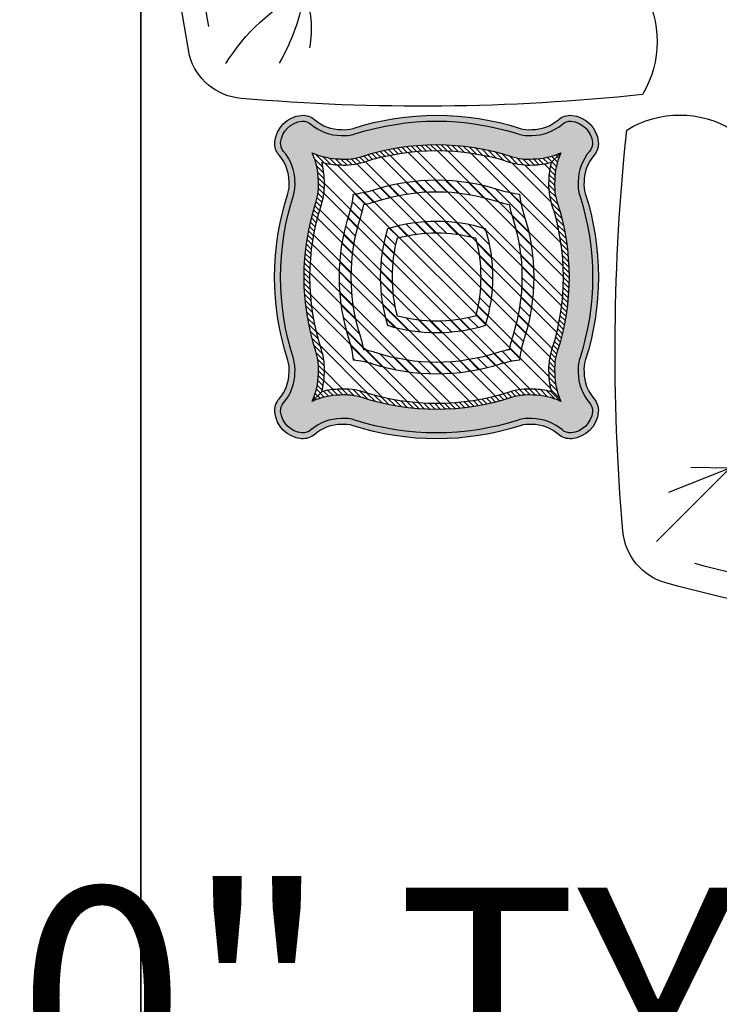
# Model space of a CAD drawing. Units: inches. Extents: x 844 to 2234, y 346 to 1084.
# Tile 5 of 93: x 1093 to 1112, y 653 to 680. Entities that reach past the tile are written whole.
import ezdxf

# ---------------------------------------------------------------- set-up
doc = ezdxf.new("R2010")
doc.units = ezdxf.units.IN
doc.header["$MEASUREMENT"] = 0
for name, color, linetype, lineweight in [('A-ANNO-DIMS', 2, 'Continuous', 18), ('A-WALL', 7, 'Continuous', 35), ('furniture', 8, 'Continuous', 18)]:
    doc.layers.add(name, color=color, linetype=linetype, lineweight=lineweight)
for name, color, linetype in [('RA-AP-01$0$FURN', 3, 'Continuous'), ('RA-AP-01$0$steel', 193, 'Continuous'), ('RA-AP-01$0$WOOD', 64, 'Continuous')]:
    doc.layers.add(name, color=color, linetype=linetype)
doc.styles.get("Standard").update_dxf_attribs({"font": 'arial.ttf'})
doc.dimstyles.get("Standard").update_dxf_attribs({"dimtxt": 6, "dimasz": 3, "dimexe": 0.18, "dimexo": 0.0625, "dimgap": 0.09, "dimtad": 0, "dimtih": 1, "dimtoh": 1, "dimdec": 1, "dimzin": 0, "dimdsep": 46, "dimlunit": 3, "dimtxsty": 'Standard', "dimblk": 'ARCHTICK', "dimcen": 0.09, "dimadec": 0, "dimazin": 0, "dimtfac": 1, "dimtdec": 1, "dimtofl": 0, "dimtmove": 0, "dimatfit": 3, "dimfxl": 1, "dimtolj": 1, "dimtzin": 0, "dimarcsym": 0})
pattern_1 = [(45, (0, 1.362436106329781), (-0.0088388347648318, 0.0088388347648318), [])]
pattern_2 = [(45, (0, 1.362436106329781), (-0.0044194173824159, 0.0044194173824159), [])]

# ---------------------------------------------------------------- blocks, each defined once
blk = doc.blocks.new('A$C2FCF5309')
at = {"layer": 'RA-AP-01$0$FURN'}
h = blk.add_hatch(dxfattribs=at)
h.set_pattern_fill('ANSI31', color=256, scale=0.1, style=0)
h.set_pattern_definition(pattern_1)
h.paths.add_polyline_path([(5.038683893313746, -5.169250834004607, -0.1583983521602212), (5.038683893312098, -5.373464580902012, 0.0306258898943267), (5.033304057242972, -5.394827569605182, 0.0306258898948892), (5.01194106853941, -5.40020740567441, -0.1028142994996694), (4.878286182323899, -5.414871334512708), (4.863600873530158, -5.43331743520547, 0.1120482678681049), (5.018059823131753, -5.419248541734471, -0.052642197802937), (5.050972078299936, -5.412495590662115, -0.0526421977994963), (5.057725029371615, -5.379583335496025, 0.1583028414702701), (5.057725029372958, -5.163132079409654, -0.052642197806903), (5.050972078299777, -5.130219824239078, -0.0526421977995126), (5.018059823133679, -5.123466873167369, 0.0215995840215353), (4.988903013548211, -5.115372132362452), (4.975007495303644, -5.132826183367946, -0.0289147572844802), (5.011941068537408, -5.142508009226167, 0.0306258898976746), (5.033304057242868, -5.147887845296027, 0.0306258899022411)])
h.paths.add_polyline_path([(4.975007495303645, -5.132826183367946), (4.988903013548211, -5.115372132362452, 0.1362374241599938), (4.801608567045604, -5.12346687316654, -0.0526421978036853), (4.768696311876971, -5.130219824239102, -0.05264219780204), (4.761943360804856, -5.163132079406747, 0.1583028414743723), (4.761943360806116, -5.379583335498449, -0.0526421977955461), (4.768696311877141, -5.412495590662114, -0.0526421978073986), (4.801608567048022, -5.419248541735437, 0.0454484293938888), (4.863600873530158, -5.43331743520547), (4.878286182323899, -5.414871334512708, -0.0546933379798044), (4.80772732164382, -5.40020740567649, 0.030625889903973), (4.786364332934043, -5.394827569605216, 0.0306258898932853), (4.780984496865101, -5.373464580902791, -0.1583983521638281), (4.780984496864308, -5.169250834000963, 0.03062588989692), (4.786364332933943, -5.147887845296004, 0.0306258898946324), (4.807727321637318, -5.142508009226805, -0.1288932573266927)])
h.paths.add_polyline_path([(4.843422214712861, -5.204945727074827, -0.0783685831716868), (4.924134454130224, -5.196727409635105), (4.939146578618322, -5.177870798323143, 0.1012675676854134), (4.827248748758957, -5.188772261120899, 0.1253648873081696), (4.820394258584192, -5.327034652050361), (4.837127701354095, -5.306015906404253, -0.0981593964869636)], flags=17)
h.paths.add_polyline_path([(4.843422214712824, -5.337769687826355, -0.0311091841722656), (4.837127701354095, -5.306015906404253), (4.820394258584193, -5.32703465205036, 0.0247727657431944), (4.827248748758908, -5.353943153780261, 0.0812754385032542), (4.916962478476905, -5.36629034358622), (4.933684093813825, -5.345286454285511, -0.0876255421014372)], flags=17)
h.paths.add_polyline_path([(4.992419641418037, -5.353943153780226, 0.1506053783834298), (4.992419641417933, -5.188772261120954, 0.0485966419124224), (4.939146578618321, -5.177870798323143), (4.924134454130224, -5.196727409635105, -0.0507799419579301), (4.976246175464031, -5.204945727074882, -0.1296645318906876), (4.97624617546411, -5.337769687826316, -0.0415667119298777), (4.933684093813825, -5.345286454285511), (4.916962478476905, -5.36629034358622, 0.0684915676023693)], flags=17)
h = blk.add_hatch(dxfattribs=at)
h.set_pattern_fill('ANSI31', color=256, scale=0.1, style=0)
h.set_pattern_definition(pattern_1)
h.paths.add_polyline_path([(5.038683893313746, -5.169250834004607, -0.1583983521602212), (5.038683893312098, -5.373464580902012, 0.0306258898943267), (5.033304057242972, -5.394827569605182, 0.0306258898948892), (5.01194106853941, -5.40020740567441, -0.1028142994996694), (4.878286182323899, -5.414871334512708), (4.863600873530158, -5.43331743520547, 0.1120482678681049), (5.018059823131753, -5.419248541734471, -0.052642197802937), (5.050972078299936, -5.412495590662115, -0.0526421977994963), (5.057725029371615, -5.379583335496025, 0.1583028414702701), (5.057725029372958, -5.163132079409654, -0.052642197806903), (5.050972078299777, -5.130219824239078, -0.0526421977995126), (5.018059823133679, -5.123466873167369, 0.0215995840215353), (4.988903013548211, -5.115372132362452), (4.975007495303644, -5.132826183367946, -0.0289147572844802), (5.011941068537408, -5.142508009226167, 0.0306258898976746), (5.033304057242868, -5.147887845296027, 0.0306258899022411)])
h.paths.add_polyline_path([(4.975007495303645, -5.132826183367946), (4.988903013548211, -5.115372132362452, 0.1362374241599938), (4.801608567045604, -5.12346687316654, -0.0526421978036853), (4.768696311876971, -5.130219824239102, -0.05264219780204), (4.761943360804856, -5.163132079406747, 0.1583028414743723), (4.761943360806116, -5.379583335498449, -0.0526421977955461), (4.768696311877141, -5.412495590662114, -0.0526421978073986), (4.801608567048022, -5.419248541735437, 0.0454484293938888), (4.863600873530158, -5.43331743520547), (4.878286182323899, -5.414871334512708, -0.0546933379798044), (4.80772732164382, -5.40020740567649, 0.030625889903973), (4.786364332934043, -5.394827569605216, 0.0306258898932853), (4.780984496865101, -5.373464580902791, -0.1583983521638281), (4.780984496864308, -5.169250834000963, 0.03062588989692), (4.786364332933943, -5.147887845296004, 0.0306258898946324), (4.807727321637318, -5.142508009226805, -0.1288932573266927)])
h.paths.add_polyline_path([(4.843422214712861, -5.204945727074827, -0.0783685831716868), (4.924134454130224, -5.196727409635105), (4.939146578618322, -5.177870798323143, 0.1012675676854134), (4.827248748758957, -5.188772261120899, 0.1253648873081696), (4.820394258584192, -5.327034652050361), (4.837127701354095, -5.306015906404253, -0.0981593964869636)], flags=17)
h.paths.add_polyline_path([(4.843422214712824, -5.337769687826355, -0.0311091841722656), (4.837127701354095, -5.306015906404253), (4.820394258584193, -5.32703465205036, 0.0247727657431944), (4.827248748758908, -5.353943153780261, 0.0812754385032542), (4.916962478476905, -5.36629034358622), (4.933684093813825, -5.345286454285511, -0.0876255421014372)], flags=17)
h.paths.add_polyline_path([(4.992419641418037, -5.353943153780226, 0.1506053783834298), (4.992419641417933, -5.188772261120954, 0.0485966419124224), (4.939146578618321, -5.177870798323143), (4.924134454130224, -5.196727409635105, -0.0507799419579301), (4.976246175464031, -5.204945727074882, -0.1296645318906876), (4.97624617546411, -5.337769687826316, -0.0415667119298777), (4.933684093813825, -5.345286454285511), (4.916962478476905, -5.36629034358622, 0.0684915676023693)], flags=17)
at = {"layer": 'RA-AP-01$0$WOOD'}
h = blk.add_hatch(color=256, dxfattribs=at)
edge = h.paths.add_edge_path()
edge.add_arc((4.683001772622394, -5.026441828662609), 0.0299999999999998, 48.77105092035535, 95.25687599427813)
edge.add_arc((4.684834195088484, -5.046357707450686), 0.0499999999998897, 95.25687599443106, 174.7431240064049)
edge.add_arc((4.664918316300367, -5.044525284985046), 0.0300000000000005, 174.7431240062535, 221.2289490796905)
edge.add_arc((4.591236830209155, -5.109094338216345), 0.0679700159630267, -0.5333070513215148, 41.228949079691915, ccw=False)
edge.add_arc((4.609451302807284, -5.114694777173187), 0.0500000000000008, -17.3556839752095, 5.7020707654044145, ccw=False)
edge.add_arc((5.095208119646659, -5.271357707450659), 0.4603971832811796, 162.0683908477609, 197.9316091523306)
edge.add_arc((4.609451302807533, -5.428020637728902), 0.0500000000000006, -5.702070765320514, 17.355683975293914, ccw=False)
edge.add_arc((4.591236830209412, -5.433621076685779), 0.0679700159630261, -41.228949079600625, 0.5333070514128053, ccw=False)
edge.add_arc((4.664918316300727, -5.498190129916959), 0.0299999999999995, 138.7710509204022, 185.256875994324)
edge.add_arc((4.684834195088642, -5.496357707450695), 0.0499999999997451, 185.2568759946742, 264.74312400432)
edge.add_arc((4.683001772622394, -5.516273586238612), 0.03, 264.743124003969, 311.2289490796446)
edge.add_arc((4.747570825853633, -5.589955072329876), 0.0679700159630271, 89.4666929486321, 131.2289490796457, ccw=False)
edge.add_arc((4.753171264810493, -5.57174059973175), 0.0500000000000015, 72.64431602474701, 95.70207076536133, ccw=False)
edge.add_arc((4.909834195088355, -5.085983782892503), 0.4603971832811774, 252.0683908477147, 287.9316091522845)
edge.add_arc((5.06649712536621, -5.57174059973175), 0.0499999999999999, 84.29792923463953, 107.35568397525361, ccw=False)
edge.add_arc((5.072097564323069, -5.589955072329877), 0.0679700159630274, 48.771050920354185, 90.5333070513679, ccw=False)
edge.add_arc((5.136666617554309, -5.516273586238614), 0.0299999999999997, 228.771050920353, 275.2568759942969)
edge.add_arc((5.134834195088338, -5.496357707450417), 0.0499999999999982, 275.2568759942949, 354.7431240057633)
edge.add_arc((5.154750073876535, -5.498190129916372), 0.0299999999999999, 354.7431240057662, 401.2289490796891)
edge.add_arc((5.228431559967749, -5.433621076685074), 0.0679700159630274, 179.4666929486771, 221.2289490796903, ccw=False)
edge.add_arc((5.210217087369615, -5.428020637728227), 0.0499999999999976, 162.6443160247947, 185.7020707654089, ccw=False)
edge.add_arc((4.724460270530244, -5.271357707450757), 0.4603971832811793, 342.0683908477607, 377.9316091523305)
edge.add_arc((5.210217087369368, -5.114694777172509), 0.0500000000000019, 174.2979292346878, 197.355683975302, ccw=False)
edge.add_arc((5.228431559967489, -5.109094338215639), 0.0679700159630279, 138.7710509203993, 180.5333070514128, ccw=False)
edge.add_arc((5.154750073876174, -5.044525284984457), 0.0300000000000001, 318.771050920401, 365.2568759954636)
edge.add_arc((5.13483419508816, -5.046357707450624), 0.0499999999998349, 5.256875995237118, 84.74312400549572)
edge.add_arc((5.136666617554308, -5.026441828662608), 0.0299999999999994, 84.74312400572185, 131.2289490796446)
edge.add_arc((5.072097564323072, -4.952760342571343), 0.0679700159630261, 269.4666929486298, 311.22894907964354, ccw=False)
edge.add_arc((5.066497125366206, -4.97097481516947), 0.0499999999999992, 252.64431602475162, 275.70207076536565, ccw=False)
edge.add_arc((4.909834195088355, -5.456731632008717), 0.4603971832811764, 72.06839084771546, 107.9316091522853)
edge.add_arc((4.753171264810493, -4.970974815169471), 0.0500000000000016, 264.2979292346387, 287.355683975253, ccw=False)
edge.add_arc((4.747570825853633, -4.952760342571346), 0.0679700159630274, 228.7710509203543, 270.5333070513679, ccw=False)
edge = h.paths.add_edge_path(flags=16)
edge.add_arc((4.683001772622395, -5.026441828662608), 0.019999999999999, 48.7710509203555, 95.2568759942793)
edge.add_arc((4.684834195088469, -5.046357707450671), 0.0399999999998731, 95.2568759944489, 174.7431240064248)
edge.add_arc((4.664918316300404, -5.044525284985035), 0.020000000000036, 174.7431240062186, 221.2289490796461)
edge.add_arc((4.591236830209151, -5.109094338216346), 0.0779700159630296, -0.13764630038667747, 41.228949079689585, ccw=False)
edge.add_arc((4.609451302807307, -5.11469477717304), 0.060000000000024, -17.406127045137907, 5.176192161068002, ccw=False)
edge.add_arc((5.09520811964665, -5.271357707450659), 0.4503971832811708, 162.0623235129628, 197.9376764869162)
edge.add_arc((4.609451302807532, -5.428020637728943), 0.0599999999999982, -5.176192160466428, 17.406127046715312, ccw=False)
edge.add_arc((4.591236830209414, -5.433621076685778), 0.0779700159630257, -41.2289490796029, 0.13764630095249686, ccw=False)
edge.add_arc((4.664918316300731, -5.498190129916961), 0.0200000000000047, 138.7710509204103, 185.2568759943212)
edge.add_arc((4.684834195088606, -5.496357707450731), 0.0399999999997066, 185.2568759947174, 264.7431240043665)
edge.add_arc((4.683001772622369, -5.516273586238541), 0.020000000000069, 264.7431240038842, 311.2289490795622)
edge.add_arc((4.747570825853635, -5.589955072329884), 0.0779700159630344, 89.8623536987642, 131.2289490796432, ccw=False)
edge.add_arc((4.753171264810603, -5.571740599731771), 0.0599999999999895, 72.5938729544394, 95.1761921602253, ccw=False)
edge.add_arc((4.909834195088365, -5.085983782892505), 0.4503971832811724, 252.0623235129989, 287.9376764870498)
edge.add_arc((5.066497125366216, -5.571740599731755), 0.0600000000000047, 84.8238078399923, 107.40612704528041, ccw=False)
edge.add_arc((5.072097564322998, -5.589955072329853), 0.077970015963056, 48.771050920303594, 90.13764630126451, ccw=False)
edge.add_arc((5.136666617554307, -5.516273586238622), 0.0199999999999931, 228.771050920344, 275.2568759943037)
edge.add_arc((5.134834195088338, -5.496357707450416), 0.0400000000000004, 275.2568759942928, 354.7431240057607)
edge.add_arc((5.154750073876533, -5.498190129916375), 0.0200000000000037, 354.7431240057783, 401.2289490796939)
edge.add_arc((5.228431559967745, -5.433621076685076), 0.0779700159630239, 179.8623536995147, 221.2289490796908, ccw=False)
edge.add_arc((5.210217087369586, -5.428020637728345), 0.0600000000000054, 162.5938729554486, 185.1761921609759, ccw=False)
edge.add_arc((4.724460270530243, -5.271357707450766), 0.4503971832811826, 342.0623235128896, 377.937676486982)
edge.add_arc((5.210217087369347, -5.114694777172486), 0.0599999999999777, 174.8238078387611, 197.4061270462219, ccw=False)
edge.add_arc((5.228431559967523, -5.109094338215542), 0.0779700159629885, 138.7710509204687, 180.1376463004423, ccw=False)
edge.add_arc((5.154750073876175, -5.044525284984459), 0.0199999999999989, 318.771050920406, 365.2568759954698)
edge.add_arc((5.134834195088138, -5.046357707450646), 0.0399999999998586, 5.256875995208452, 84.74312400546732)
edge.add_arc((5.136666617554292, -5.02644182866256), 0.0199999999999529, 84.74312400577769, 131.2289490797025)
edge.add_arc((5.072097564323069, -4.952760342571338), 0.077970015963032, 269.86235369901414, 311.2289490796421, ccw=False)
edge.add_arc((5.06649712536618, -4.97097481516946), 0.0600000000000007, 252.5938729548277, 275.17619216047467, ccw=False)
edge.add_arc((4.909834195088353, -5.456731632008716), 0.4503971832811739, 72.06232351293887, 107.9376764867365)
edge.add_arc((4.753171264810429, -4.970974815169467), 0.0599999999999991, 264.82380783985815, 287.40612704769893, ccw=False)
edge.add_arc((4.747570825853681, -4.952760342571361), 0.0779700159630467, 228.7710509203206, 270.13764630113724, ccw=False)
h = blk.add_hatch(color=256, dxfattribs=at)
edge = h.paths.add_edge_path()
edge.add_arc((4.683001772622395, -5.026441828662608), 0.019999999999999, 48.7710509203555, 95.2568759942793)
edge.add_arc((4.684834195088469, -5.046357707450671), 0.0399999999998731, 95.2568759944489, 174.7431240064248)
edge.add_arc((4.664918316300404, -5.044525284985035), 0.020000000000036, 174.7431240062186, 221.2289490796461)
edge.add_arc((4.591236830209151, -5.109094338216346), 0.0779700159630296, -0.13764630038667747, 41.228949079689585, ccw=False)
edge.add_arc((4.609451302807307, -5.11469477717304), 0.060000000000024, -17.406127045137907, 5.176192161068002, ccw=False)
edge.add_arc((5.09520811964665, -5.271357707450659), 0.4503971832811708, 162.0623235129628, 197.9376764869162)
edge.add_arc((4.609451302807532, -5.428020637728943), 0.0599999999999982, -5.176192160466428, 17.406127046715312, ccw=False)
edge.add_arc((4.591236830209414, -5.433621076685778), 0.0779700159630257, -41.2289490796029, 0.13764630095249686, ccw=False)
edge.add_arc((4.664918316300731, -5.498190129916961), 0.0200000000000047, 138.7710509204103, 185.2568759943212)
edge.add_arc((4.684834195088606, -5.496357707450731), 0.0399999999997066, 185.2568759947174, 264.7431240043665)
edge.add_arc((4.683001772622369, -5.516273586238541), 0.020000000000069, 264.7431240038842, 311.2289490795622)
edge.add_arc((4.747570825853635, -5.589955072329884), 0.0779700159630344, 89.8623536987642, 131.2289490796432, ccw=False)
edge.add_arc((4.753171264810603, -5.571740599731771), 0.0599999999999895, 72.5938729544394, 95.1761921602253, ccw=False)
edge.add_arc((4.909834195088365, -5.085983782892505), 0.4503971832811724, 252.0623235129989, 287.9376764870498)
edge.add_arc((5.066497125366216, -5.571740599731755), 0.0600000000000047, 84.8238078399923, 107.40612704528041, ccw=False)
edge.add_arc((5.072097564322998, -5.589955072329853), 0.077970015963056, 48.771050920303594, 90.13764630126451, ccw=False)
edge.add_arc((5.136666617554307, -5.516273586238622), 0.0199999999999931, 228.771050920344, 275.2568759943037)
edge.add_arc((5.134834195088338, -5.496357707450416), 0.0400000000000004, 275.2568759942928, 354.7431240057607)
edge.add_arc((5.154750073876533, -5.498190129916375), 0.0200000000000037, 354.7431240057783, 401.2289490796939)
edge.add_arc((5.228431559967745, -5.433621076685076), 0.0779700159630239, 179.8623536995147, 221.2289490796908, ccw=False)
edge.add_arc((5.210217087369586, -5.428020637728345), 0.0600000000000054, 162.5938729554486, 185.1761921609759, ccw=False)
edge.add_arc((4.724460270530243, -5.271357707450766), 0.4503971832811826, 342.0623235128896, 377.937676486982)
edge.add_arc((5.210217087369347, -5.114694777172486), 0.0599999999999777, 174.8238078387611, 197.4061270462219, ccw=False)
edge.add_arc((5.228431559967523, -5.109094338215542), 0.0779700159629885, 138.7710509204687, 180.1376463004423, ccw=False)
edge.add_arc((5.154750073876175, -5.044525284984459), 0.0199999999999989, 318.771050920406, 365.2568759954698)
edge.add_arc((5.134834195088138, -5.046357707450646), 0.0399999999998586, 5.256875995208452, 84.74312400546732)
edge.add_arc((5.136666617554292, -5.02644182866256), 0.0199999999999529, 84.74312400577769, 131.2289490797025)
edge.add_arc((5.072097564323069, -4.952760342571338), 0.077970015963032, 269.86235369901414, 311.2289490796421, ccw=False)
edge.add_arc((5.06649712536618, -4.97097481516946), 0.0600000000000007, 252.5938729548277, 275.17619216047467, ccw=False)
edge.add_arc((4.909834195088353, -5.456731632008716), 0.4503971832811739, 72.06232351293887, 107.9376764867365)
edge.add_arc((4.753171264810429, -4.970974815169467), 0.0599999999999991, 264.82380783985815, 287.40612704769893, ccw=False)
edge.add_arc((4.747570825853681, -4.952760342571361), 0.0779700159630467, 228.7710509203206, 270.13764630113724, ccw=False)
edge = h.paths.add_edge_path(flags=16)
edge.add_arc((4.591236830209151, -5.109094338216348), 0.1179700159630308, 0.7417751874182841, 24.563326950263672, ccw=False)
edge.add_arc((4.609451302807302, -5.114694777173093), 0.100000000000012, -17.52836504564658, 4.087328884225087, ccw=False)
edge.add_arc((5.095208119646651, -5.271357707450657), 0.4103971832811724, 162.0403002448777, 197.9596997550675)
edge.add_arc((4.60945130280753, -5.428020637728918), 0.1000000000000027, -4.087328883827581, 17.528365046291924, ccw=False)
edge.add_arc((4.591236830209414, -5.433621076685779), 0.1179700159630246, 335.43667305041845, 359.2582248129738, ccw=False)
edge.add_arc((4.747570825853596, -5.589955072329891), 0.117970015963042, 90.7417751868461, 114.5633269496104, ccw=False)
edge.add_arc((4.753171264810559, -5.571740599731767), 0.0999999999999976, 72.47163495370341, 94.0873288836737, ccw=False)
edge.add_arc((4.909834195088367, -5.085983782892503), 0.4103971832811735, 252.0403002449999, 287.9596997551833)
edge.add_arc((5.066497125366205, -5.571740599731755), 0.1000000000000057, 85.91267111645209, 107.5283650455624, ccw=False)
edge.add_arc((5.072097564322985, -5.58995507232986), 0.117970015963046, 65.4366730497672, 89.25822481317113, ccw=False)
edge.add_arc((5.22843155996773, -5.433621076684992), 0.1179700159630096, 180.7417751873964, 204.5633269502712, ccw=False)
edge.add_arc((5.210217087369591, -5.428020637728301), 0.0999999999999969, 162.4716349546276, 184.0873288841682, ccw=False)
edge.add_arc((4.724460270530243, -5.271357707450766), 0.4103971832811825, 342.0403002448147, 377.9596997550345)
edge.add_arc((5.210217087369347, -5.114694777172489), 0.0999999999999796, 175.9126711156995, 197.5283650464392, ccw=False)
edge.add_arc((5.228431559967512, -5.109094338215525), 0.1179700159630019, 155.4366730502992, 179.2582248126247, ccw=False)
edge.add_arc((5.072097564323172, -4.952760342571314), 0.1179700159630537, 270.74177518697286, 294.56332694975765, ccw=False)
edge.add_arc((5.066497125366189, -4.970974815169462), 0.1000000000000017, 252.471634954247, 274.0873288838353, ccw=False)
edge.add_arc((4.909834195088353, -5.456731632008716), 0.4103971832811758, 72.04030024486342, 107.9596997549354)
edge.add_arc((4.75317126481046, -4.970974815169467), 0.1000000000000041, 265.91267111635307, 287.5283650466103, ccw=False)
edge.add_arc((4.747570825853629, -4.952760342571342), 0.1179700159630538, 245.43667304992562, 269.2582248131125, ccw=False)
h = blk.add_hatch(dxfattribs=at)
h.set_pattern_fill('ANSI31', color=256, scale=0.05, style=0)
h.set_pattern_definition(pattern_2)
h.paths.add_polyline_path([(5.105336294329346, -5.394854099602528, 0.0940138826956367), (5.100476366643778, -5.435568764288975, 0.0606271852326483), (5.104678567100611, -5.466202079462671, 0.0606271852344644), (5.074045251925975, -5.46199987900586, 0.0940138827021426), (5.033330587236848, -5.466859806692645, -0.1305325492494615), (4.828072633169377, -5.477944178050054), (4.821119726105699, -5.486677669841435, 0.1336226599878005), (5.036379334063467, -5.476383803188216, -0.0945969211935747), (5.073624810952389, -5.471994942692536, -0.1043170707892296), (5.121137550891356, -5.48266106325342, -0.1043170707868944), (5.110471430330457, -5.435148323315565, -0.0945969211952573), (5.114860290825935, -5.397902846425963, 0.1580239521433527), (5.114860290826324, -5.144812568476775, -0.0945969212010491), (5.110471430330247, -5.10756709158498, -0.1043170707844371), (5.121137550890657, -5.060054351648168, -0.104317070786514), (5.073624810952866, -5.070720472208642, -0.0945969211958523), (5.036379334063063, -5.066331611712874, 0.1580239521426795), (4.783289056114906, -5.066331611712465, -0.0945969211985319), (4.746043579224103, -5.070720472208672, -0.1043170707882665), (4.698530839285552, -5.060054351647925, -0.1043170707867205), (4.709196959846443, -5.10756709158571, -0.094596921196788), (4.704808099350826, -5.144812568475902, 0.1580239521433127), (4.704808099350699, -5.397902846425022, -0.094596921197841), (4.709196959846712, -5.435148323315576, -0.1043170707855109), (4.698530839286393, -5.482661063252921, -0.1043170707864168), (4.746043579224162, -5.471994942692571, -0.0945969211977586), (4.783289056114671, -5.476383803188671, 0.0238966994662183), (4.821119726105699, -5.486677669841435), (4.828072633169378, -5.477944178050054, -0.0269814195959459), (4.786337802940177, -5.466859806692736, 0.0940138827039629), (4.745623138250268, -5.461999879005895, 0.0606271852320776), (4.714989823076826, -5.466202079462476, 0.0606271852304618), (4.719192023533341, -5.435568764289856, 0.0940138826917763), (4.714332095848404, -5.394854099604977, -0.1580706864542086), (4.714332095846561, -5.147861315302034, 0.0940138827032017), (4.719192023533127, -5.107146650612438, 0.0606271852329446), (4.714989823076289, -5.076513335438588, 0.0606271852340035), (4.745623138250698, -5.08071553589536, 0.0940138827025969), (4.786337802940015, -5.075855608208526, -0.1580706864508517), (5.033330587237968, -5.075855608208939, 0.0940138827009578), (5.074045251926627, -5.080715535895319, 0.0606271852322557), (5.104678567100159, -5.076513335438697, 0.0606271852308743), (5.100476366643561, -5.107146650611519, 0.0940138827178109), (5.105336294331983, -5.147861315307182, -0.1580706864490946)])
h = blk.add_hatch(dxfattribs=at)
h.set_pattern_fill('ANSI31', color=256, scale=0.05, style=0)
h.set_pattern_definition(pattern_2)
h.paths.add_polyline_path([(5.105336294329346, -5.394854099602528, 0.0940138826956367), (5.100476366643778, -5.435568764288975, 0.0606271852326483), (5.104678567100611, -5.466202079462671, 0.0606271852344644), (5.074045251925975, -5.46199987900586, 0.0940138827021426), (5.033330587236848, -5.466859806692645, -0.1305325492494615), (4.828072633169377, -5.477944178050054), (4.821119726105699, -5.486677669841435, 0.1336226599878005), (5.036379334063467, -5.476383803188216, -0.0945969211935747), (5.073624810952389, -5.471994942692536, -0.1043170707892296), (5.121137550891356, -5.48266106325342, -0.1043170707868944), (5.110471430330457, -5.435148323315565, -0.0945969211952573), (5.114860290825935, -5.397902846425963, 0.1580239521433527), (5.114860290826324, -5.144812568476775, -0.0945969212010491), (5.110471430330247, -5.10756709158498, -0.1043170707844371), (5.121137550890657, -5.060054351648168, -0.104317070786514), (5.073624810952866, -5.070720472208642, -0.0945969211958523), (5.036379334063063, -5.066331611712874, 0.1580239521426795), (4.783289056114906, -5.066331611712465, -0.0945969211985319), (4.746043579224103, -5.070720472208672, -0.1043170707882665), (4.698530839285552, -5.060054351647925, -0.1043170707867205), (4.709196959846443, -5.10756709158571, -0.094596921196788), (4.704808099350826, -5.144812568475902, 0.1580239521433127), (4.704808099350699, -5.397902846425022, -0.094596921197841), (4.709196959846712, -5.435148323315576, -0.1043170707855109), (4.698530839286393, -5.482661063252921, -0.1043170707864168), (4.746043579224162, -5.471994942692571, -0.0945969211977586), (4.783289056114671, -5.476383803188671, 0.0238966994662183), (4.821119726105699, -5.486677669841435), (4.828072633169378, -5.477944178050054, -0.0269814195959459), (4.786337802940177, -5.466859806692736, 0.0940138827039629), (4.745623138250268, -5.461999879005895, 0.0606271852320776), (4.714989823076826, -5.466202079462476, 0.0606271852304618), (4.719192023533341, -5.435568764289856, 0.0940138826917763), (4.714332095848404, -5.394854099604977, -0.1580706864542086), (4.714332095846561, -5.147861315302034, 0.0940138827032017), (4.719192023533127, -5.107146650612438, 0.0606271852329446), (4.714989823076289, -5.076513335438588, 0.0606271852340035), (4.745623138250698, -5.08071553589536, 0.0940138827025969), (4.786337802940015, -5.075855608208526, -0.1580706864508517), (5.033330587237968, -5.075855608208939, 0.0940138827009578), (5.074045251926627, -5.080715535895319, 0.0606271852322557), (5.104678567100159, -5.076513335438697, 0.0606271852308743), (5.100476366643561, -5.107146650611519, 0.0940138827178109), (5.105336294331983, -5.147861315307182, -0.1580706864490946)])
h = blk.add_hatch(dxfattribs=at)
h.set_pattern_fill('ANSI32,_I', color=256, scale=0.1, style=2)
h.set_pattern_definition([(45, (0, 0), (-0.0265165042944955, 0.0265165042944955), []), (45, (0.0176776695, 0), (-0.0265165042944955, 0.0265165042944955), [])])
h.paths.add_polyline_path([(4.843422214712824, -5.337769687826354, 0.1296645318905289), (4.97624617546411, -5.337769687826316, 0.1296645318906876), (4.976246175464032, -5.204945727074882, 0.129664531890418), (4.843422214712861, -5.204945727074827, 0.129664531890765)], flags=0)
h.paths.add_polyline_path([(5.039131224122924, -5.170637849998464, -0.0326520429852175), (5.033304057242868, -5.147887845296027, -0.0326520429894721), (5.010554052537512, -5.142060678415043, 0.1561383235202698), (4.809114337641437, -5.142060678414318, -0.0326520429925972), (4.786364332933944, -5.147887845296004, -0.0326520429914489), (4.780537166052582, -5.170637850002729, 0.1561383235189577), (4.780537166052134, -5.37207756489719, -0.0326520429934175), (4.786364332934042, -5.394827569605215, -0.0326520429823496), (4.809114337634529, -5.400654736484653, 0.156138323524066), (5.010554052535268, -5.400654736486903, -0.032652042992888), (5.033304057242972, -5.394827569605183, -0.0326520429928733), (5.039131224124712, -5.372077564897496, 0.1561383235226786)], flags=0)
h.paths.add_polyline_path([(4.992419641418037, -5.353943153780226, -0.1506053783832862), (4.827248748758909, -5.353943153780261, -0.1506053783835069), (4.827248748758957, -5.188772261120899, -0.1506053783831346), (4.992419641417933, -5.188772261120954, -0.1506053783834298)], flags=0)
h.paths.add_polyline_path([(4.976246175464111, -5.337769687826316, -0.1296645318905298), (4.843422214712824, -5.337769687826354, -0.129664531890765), (4.843422214712862, -5.204945727074827, -0.1296645318904162), (4.976246175464031, -5.204945727074882, -0.1296645318906876)], flags=0)
h.paths.add_polyline_path([(5.105721254232479, -5.149054940982025, -0.0968902512052664), (5.100476366643561, -5.107146650611519, -0.0606271852308743), (5.104678567100159, -5.076513335438697, -0.0606271852322574), (5.074045251926626, -5.080715535895319, -0.0968902512197216), (5.032136961550132, -5.075470648304253, 0.1564657949319774), (4.787531428625239, -5.075470648304682, -0.0968902512150626), (4.745623138250699, -5.08071553589536, -0.060627185234009), (4.714989823076288, -5.076513335438587, -0.0606271852329501), (4.719192023533127, -5.10714665061244, -0.0968902512185585), (4.713947135942331, -5.149054940988458, 0.1564657949285579), (4.713947135940853, -5.393660473908259, -0.0968902512319826), (4.71919202353334, -5.435568764289873, -0.0606271852304288), (4.714989823076825, -5.466202079462476, -0.0606271852320811), (4.745623138250269, -5.461999879005895, -0.0968902512162649), (4.787531428625332, -5.467244766596559, 0.1564657949327057), (5.032136961551311, -5.46724476659659, -0.0968902512153659), (5.074045251925975, -5.46199987900586, -0.0606271852344627), (5.10467856710061, -5.466202079462671, -0.0606271852326483), (5.100476366643777, -5.435568764288975, -0.0968902512258216), (5.105721254235559, -5.393660473909953, 0.1564657949340142)])
h.paths.add_polyline_path([(5.057725029371625, -5.379583335495999, 0.0526421977995391), (5.050972078299936, -5.412495590662114, 0.0526421978029782), (5.018059823131728, -5.419248541734479, -0.1583028414681072), (4.801608567048168, -5.419248541735485, 0.0526421978076402), (4.76869631187714, -5.412495590662113, 0.0526421977956189), (4.761943360806101, -5.379583335498404, -0.1583028414743129), (4.761943360804846, -5.163132079406778, 0.0526421978020944), (4.768696311876972, -5.130219824239101, 0.0526421978033651), (4.80160856704541, -5.123466873166602, -0.1583028414716875), (5.018059823133628, -5.123466873167353, 0.0526421977995944), (5.050972078299776, -5.130219824239078, 0.0526421978070423), (5.057725029372986, -5.163132079409739, -0.1583028414701848)], flags=16)
h.paths.add_polyline_path([(5.038683893312112, -5.373464580901968, 0.0306258898943915), (5.033304057242972, -5.394827569605182, 0.0306258898948892), (5.01194106853941, -5.40020740567441, -0.1583983521587032), (4.807727321643864, -5.400207405676503, 0.0306258899040366), (4.786364332934043, -5.394827569605215, 0.0306258898931986), (4.780984496865119, -5.37346458090285, -0.1583983521638542), (4.7809844968643, -5.169250834000989, 0.0306258898969596), (4.786364332933945, -5.147887845296004, 0.0306258898946195), (4.807727321637311, -5.142508009226808, -0.1583983521623412), (5.011941068537318, -5.142508009226139, 0.030625889897807), (5.033304057242868, -5.147887845296028, 0.0306258899020632), (5.038683893313706, -5.169250834004486, -0.1583983521602835)], flags=0)
for p, q in [((4.714989823076289, -5.076513335438588), (4.698530839285552, -5.060054351647925)), ((4.714989823076289, -5.076513335438588), (4.698530839285552, -5.060054351647925)), ((5.104678567100159, -5.076513335438697), (5.121137550890656, -5.060054351648169)), ((5.104678567100159, -5.076513335438697), (5.121137550890656, -5.060054351648169)), ((5.10467856710061, -5.466202079462671), (5.121137550891355, -5.482661063253419)), ((5.10467856710061, -5.466202079462671), (5.121137550891355, -5.482661063253419))]:
    blk.add_line(p, q, dxfattribs=at)
for points in [[(4.702773858784635, -5.003879368495489, 0.2056608120285223), (4.680253138923443, -4.996568010480312, 0.3614336704708569), (4.635044498118043, -5.041776651286372, 0.2056608120263112), (4.642355856133262, -5.064297371147306, -0.1842662638101064), (4.65920390179375, -5.10972699154053, -0.1009492694051416), (4.657174869772992, -5.129609908955028, 0.1577727036674954), (4.657174869773219, -5.41310550594699, -0.1009492694051416), (4.659203901794006, -5.432988423361486, -0.1842662638101064), (4.64235585613359, -5.478418043754737, 0.2056608120285221), (4.635044498118431, -5.500938763615934, 0.3614336704593693), (4.680253138922529, -5.546147404420826, 0.2056608120364936), (4.702773858784635, -5.538836046405732, -0.1842662638101064), (4.748203479177874, -5.52198800074528, -0.1009492694051415), (4.768086396592371, -5.524017032766053, 0.1577727036674954), (5.051581993584332, -5.524017032766055, -0.1009492694051416), (5.071464910998829, -5.521988000745282, -0.1842662638101064), (5.116894531392067, -5.538836046405734, 0.2056608120286145), (5.13941525125327, -5.546147404420911, 0.3614336704683636), (5.184623892058835, -5.500938763615299, 0.2056608120285223), (5.177312534043641, -5.478418043754112, -0.1842662638101063), (5.160464488383153, -5.432988423360887, -0.1009492694051416), (5.162493520403909, -5.41310550594639, 0.1577727036674954), (5.162493520403684, -5.129609908954428, -0.1009492694051416), (5.160464488382894, -5.109726991539933, -0.1842662638101064), (5.17731253404331, -5.064297371146681, 0.2056608120337072), (5.184623892058415, -5.041776651284888, 0.3614336704623863), (5.139415251253259, -4.99656801048031, 0.2056608120285223), (5.116894531392067, -5.003879368495487, -0.1842662638101064), (5.071464910998829, -5.020727414155937, -0.1009492694051416), (5.051581993584332, -5.018698382135166, 0.1577727036674956), (4.768086396592371, -5.018698382135168, -0.1009492694051416), (4.748203479177874, -5.020727414155941, -0.1842662638101064)], [(4.702773858784635, -5.003879368495489, 0.2056608120285223), (4.680253138923443, -4.996568010480312, 0.3614336704708569), (4.635044498118043, -5.041776651286372, 0.2056608120263112), (4.642355856133262, -5.064297371147306, -0.1842662638101064), (4.65920390179375, -5.10972699154053, -0.1009492694051416), (4.657174869772992, -5.129609908955028, 0.1577727036674954), (4.657174869773219, -5.41310550594699, -0.1009492694051416), (4.659203901794006, -5.432988423361486, -0.1842662638101064), (4.64235585613359, -5.478418043754737, 0.2056608120285221), (4.635044498118431, -5.500938763615934, 0.3614336704593693), (4.680253138922529, -5.546147404420826, 0.2056608120364936), (4.702773858784635, -5.538836046405732, -0.1842662638101064), (4.748203479177874, -5.52198800074528, -0.1009492694051415), (4.768086396592371, -5.524017032766053, 0.1577727036674954), (5.051581993584332, -5.524017032766055, -0.1009492694051416), (5.071464910998829, -5.521988000745282, -0.1842662638101064), (5.116894531392067, -5.538836046405734, 0.2056608120286145), (5.13941525125327, -5.546147404420911, 0.3614336704683636), (5.184623892058835, -5.500938763615299, 0.2056608120285223), (5.177312534043641, -5.478418043754112, -0.1842662638101063), (5.160464488383153, -5.432988423360887, -0.1009492694051416), (5.162493520403909, -5.41310550594639, 0.1577727036674954), (5.162493520403684, -5.129609908954428, -0.1009492694051416), (5.160464488382894, -5.109726991539933, -0.1842662638101064), (5.17731253404331, -5.064297371146681, 0.2056608120337072), (5.184623892058415, -5.041776651284888, 0.3614336704623863), (5.139415251253259, -4.99656801048031, 0.2056608120285223), (5.116894531392067, -5.003879368495487, -0.1842662638101064), (5.071464910998829, -5.020727414155937, -0.1009492694051416), (5.051581993584332, -5.018698382135166, 0.1577727036674956), (4.768086396592371, -5.018698382135168, -0.1009492694051416), (4.748203479177874, -5.020727414155941, -0.1842662638101064)], [(4.696183163397222, -5.011400188551196, 0.2056608120285295), (4.681169350156427, -5.006525949874411, 0.3614336704708588), (4.645002437512154, -5.042692862519237, 0.2056608120262659), (4.649876676188964, -5.057706675759887, -0.182481815856965), (4.669206621172843, -5.109281651732388, -0.0988540857970112), (4.666703803477437, -5.13264334722805, 0.1578269695851905), (4.666703803477144, -5.410072067672365, -0.0988540858013112), (4.6692066211731, -5.433433763168966, -0.1824818158591246), (4.649876676189301, -5.485008739142145, 0.2056608120284717), (4.64500243751253, -5.500022552382944, 0.3614336704593821), (4.681169350155757, -5.536189465026749, 0.2056608120365057), (4.696183163397221, -5.531315226350026, -0.1824818158605826), (4.747758139370833, -5.51198528136619, -0.0988540857951607), (4.771119834866025, -5.514488099061806, 0.1578269695856264), (5.04854855531107, -5.514488099061688, -0.0988540857929677), (5.071910250805761, -5.511985281366138, -0.1824818158609529), (5.123485226779481, -5.531315226350027, 0.2056608120286893), (5.138499040020282, -5.536189465026812, 0.3614336704683556), (5.174665952664737, -5.500022552382323, 0.2056608120284882), (5.169791713987938, -5.485008739141532, -0.1824818158574124), (5.150461769004059, -5.4334337631689, -0.0988540857940221), (5.152964586699289, -5.410072067673927, 0.1578269695858123), (5.1529645866996, -5.132643347228565, -0.0988540858025403), (5.150461769003872, -5.109281651731659, -0.1824818158565006), (5.169791713987599, -5.057706675759273, 0.2056608120337192), (5.174665952664335, -5.042692862518078, 0.3614336704623903), (5.138499040020236, -5.006525949874406, 0.2056608120285323), (5.123485226779481, -5.011400188551195, -0.1824818158594503), (5.071910250806212, -5.03073013353503, -0.09885408579455), (5.048548555311143, -5.028227315839558, 0.1578269695844942), (4.771119834867991, -5.028227315838772, -0.0988540858042156), (4.747758139370745, -5.030730133535067, -0.1824818158603032)], [(4.696183163397222, -5.011400188551196, 0.2056608120285295), (4.681169350156427, -5.006525949874411, 0.3614336704708588), (4.645002437512154, -5.042692862519237, 0.2056608120262659), (4.649876676188964, -5.057706675759887, -0.182481815856965), (4.669206621172843, -5.109281651732388, -0.0988540857970112), (4.666703803477437, -5.13264334722805, 0.1578269695851905), (4.666703803477144, -5.410072067672365, -0.0988540858013112), (4.6692066211731, -5.433433763168966, -0.1824818158591246), (4.649876676189301, -5.485008739142145, 0.2056608120284717), (4.64500243751253, -5.500022552382944, 0.3614336704593821), (4.681169350155757, -5.536189465026749, 0.2056608120365057), (4.696183163397221, -5.531315226350026, -0.1824818158605826), (4.747758139370833, -5.51198528136619, -0.0988540857951607), (4.771119834866025, -5.514488099061806, 0.1578269695856264), (5.04854855531107, -5.514488099061688, -0.0988540857929677), (5.071910250805761, -5.511985281366138, -0.1824818158609529), (5.123485226779481, -5.531315226350027, 0.2056608120286893), (5.138499040020282, -5.536189465026812, 0.3614336704683556), (5.174665952664737, -5.500022552382323, 0.2056608120284882), (5.169791713987938, -5.485008739141532, -0.1824818158574124), (5.150461769004059, -5.4334337631689, -0.0988540857940221), (5.152964586699289, -5.410072067673927, 0.1578269695858123), (5.1529645866996, -5.132643347228565, -0.0988540858025403), (5.150461769003872, -5.109281651731659, -0.1824818158565006), (5.169791713987599, -5.057706675759273, 0.2056608120337192), (5.174665952664335, -5.042692862518078, 0.3614336704623903), (5.138499040020236, -5.006525949874406, 0.2056608120285323), (5.123485226779481, -5.011400188551195, -0.1824818158594503), (5.071910250806212, -5.03073013353503, -0.09885408579455), (5.048548555311143, -5.028227315839558, 0.1578269695844942), (4.771119834867991, -5.028227315838772, -0.0988540858042156), (4.747758139370745, -5.030730133535067, -0.1824818158603032)], [(4.698530839285552, -5.060054351647925, -0.1043170707867612), (4.709196959846444, -5.107567091585729, -0.0945969211969405), (4.704808099350802, -5.144812568475978, 0.1580239521432241), (4.704808099350681, -5.397902846424963, -0.0945969211980322), (4.709196959846711, -5.43514832331559, -0.104317070785482), (4.698530839286393, -5.482661063252921, -0.1043170707864036), (4.746043579224155, -5.471994942692571, -0.094596921197375), (4.78328905611452, -5.476383803188623, 0.1580239521431959), (5.036379334063463, -5.476383803188218, -0.0945969211935888), (5.07362481095239, -5.471994942692536, -0.1043170707892253), (5.121137550891355, -5.482661063253419, -0.1043170707868921), (5.110471430330457, -5.435148323315565, -0.0945969211954828), (5.114860290825962, -5.397902846425878, 0.158023952143358), (5.114860290826295, -5.144812568476682, -0.0945969212007617), (5.110471430330247, -5.107567091584995, -0.1043170707844689), (5.121137550890656, -5.060054351648169, -0.1043170707864946), (5.073624810952874, -5.070720472208642, -0.0945969211956941), (5.036379334063131, -5.066331611712896, 0.1580239521426976), (4.783289056114946, -5.066331611712452, -0.0945969211986379), (4.746043579224103, -5.070720472208672, -0.1043170707882684)], [(4.698530839285552, -5.060054351647925, -0.1043170707867612), (4.709196959846444, -5.107567091585729, -0.0945969211969405), (4.704808099350802, -5.144812568475978, 0.1580239521432241), (4.704808099350681, -5.397902846424963, -0.0945969211980322), (4.709196959846711, -5.43514832331559, -0.104317070785482), (4.698530839286393, -5.482661063252921, -0.1043170707864036), (4.746043579224155, -5.471994942692571, -0.094596921197375), (4.78328905611452, -5.476383803188623, 0.1580239521431959), (5.036379334063463, -5.476383803188218, -0.0945969211935888), (5.07362481095239, -5.471994942692536, -0.1043170707892253), (5.121137550891355, -5.482661063253419, -0.1043170707868921), (5.110471430330457, -5.435148323315565, -0.0945969211954828), (5.114860290825962, -5.397902846425878, 0.158023952143358), (5.114860290826295, -5.144812568476682, -0.0945969212007617), (5.110471430330247, -5.107567091584995, -0.1043170707844689), (5.121137550890656, -5.060054351648169, -0.1043170707864946), (5.073624810952874, -5.070720472208642, -0.0945969211956941), (5.036379334063131, -5.066331611712896, 0.1580239521426976), (4.783289056114946, -5.066331611712452, -0.0945969211986379), (4.746043579224103, -5.070720472208672, -0.1043170707882684)], [(4.714989823076289, -5.076513335438588, -0.0606271852329464), (4.719192023533127, -5.107146650612439, -0.0940138827030756), (4.714332095846578, -5.147861315301983, 0.1580706864542707), (4.714332095848417, -5.394854099605018, -0.0940138826916965), (4.719192023533341, -5.435568764289864, -0.0606271852304462), (4.714989823076826, -5.466202079462476, -0.0606271852320585), (4.745623138250258, -5.461999879005895, -0.0940138827037036), (4.786337802940059, -5.466859806692699, 0.1580706864500221), (5.033330587236783, -5.466859806692666, -0.0940138827023111), (5.074045251925979, -5.46199987900586, -0.060627185234454), (5.10467856710061, -5.466202079462671, -0.0606271852326709), (5.100476366643777, -5.435568764288963, -0.0940138826958686), (5.105336294329379, -5.394854099602421, 0.1580706864489859), (5.105336294331999, -5.147861315307237, -0.0940138827179432), (5.100476366643561, -5.107146650611518, -0.0606271852308726), (5.104678567100159, -5.076513335438697, -0.0606271852322592), (5.074045251926625, -5.080715535895319, -0.094013882701022), (5.03333058723794, -5.075855608208931, 0.1580706864508015), (4.786337802940061, -5.075855608208511, -0.0940138827027143), (4.745623138250695, -5.08071553589536, -0.0606271852339983)], [(4.714989823076289, -5.076513335438588, -0.0606271852329464), (4.719192023533127, -5.107146650612439, -0.0940138827030756), (4.714332095846578, -5.147861315301983, 0.1580706864542707), (4.714332095848417, -5.394854099605018, -0.0940138826916965), (4.719192023533341, -5.435568764289864, -0.0606271852304462), (4.714989823076826, -5.466202079462476, -0.0606271852320585), (4.745623138250258, -5.461999879005895, -0.0940138827037036), (4.786337802940059, -5.466859806692699, 0.1580706864500221), (5.033330587236783, -5.466859806692666, -0.0940138827023111), (5.074045251925979, -5.46199987900586, -0.060627185234454), (5.10467856710061, -5.466202079462671, -0.0606271852326709), (5.100476366643777, -5.435568764288963, -0.0940138826958686), (5.105336294329379, -5.394854099602421, 0.1580706864489859), (5.105336294331999, -5.147861315307237, -0.0940138827179432), (5.100476366643561, -5.107146650611518, -0.0606271852308726), (5.104678567100159, -5.076513335438697, -0.0606271852322592), (5.074045251926625, -5.080715535895319, -0.094013882701022), (5.03333058723794, -5.075855608208931, 0.1580706864508015), (4.786337802940061, -5.075855608208511, -0.0940138827027143), (4.745623138250695, -5.08071553589536, -0.0606271852339983)], [(4.768696311876972, -5.130219824239102, -0.0526421978019087), (4.761943360804882, -5.163132079406667, 0.1583028414744761), (4.761943360806133, -5.379583335498504, -0.0526421977954539), (4.76869631187714, -5.412495590662113, -0.0526421978076619), (4.801608567048181, -5.419248541735488, 0.1583028414681522), (5.0180598231318, -5.419248541734456, -0.0526421978028585), (5.050972078299936, -5.412495590662114, -0.0526421977992923), (5.057725029371576, -5.379583335496149, 0.1583028414703719), (5.057725029372956, -5.163132079409646, -0.0526421978068888), (5.050972078299776, -5.130219824239078, -0.052642197799403), (5.018059823133745, -5.12346687316739, 0.1583028414717216), (4.801608567045482, -5.123466873166579, -0.0526421978034837)], [(4.768696311876972, -5.130219824239102, -0.0526421978019087), (4.761943360804882, -5.163132079406667, 0.1583028414744761), (4.761943360806133, -5.379583335498504, -0.0526421977954539), (4.76869631187714, -5.412495590662113, -0.0526421978076619), (4.801608567048181, -5.419248541735488, 0.1583028414681522), (5.0180598231318, -5.419248541734456, -0.0526421978028585), (5.050972078299936, -5.412495590662114, -0.0526421977992923), (5.057725029371576, -5.379583335496149, 0.1583028414703719), (5.057725029372956, -5.163132079409646, -0.0526421978068888), (5.050972078299776, -5.130219824239078, -0.052642197799403), (5.018059823133745, -5.12346687316739, 0.1583028414717216), (4.801608567045482, -5.123466873166579, -0.0526421978034837)], [(4.786364332933944, -5.147887845296004, -0.0306258898969254), (4.780984496864308, -5.169250834000966, 0.1583983521638412), (4.780984496865107, -5.373464580902811, -0.0306258898932568), (4.786364332934043, -5.394827569605216, -0.0306258899041339), (4.80772732164393, -5.400207405676526, 0.1583983521586416), (5.011941068539401, -5.400207405674413, -0.0306258898949021), (5.033304057242972, -5.394827569605182, -0.0306258898943513), (5.038683893312104, -5.373464580901996, 0.1583983521602784), (5.038683893313717, -5.16925083400452, -0.0306258899021139), (5.033304057242868, -5.147887845296027, -0.030625889897777), (5.011941068537338, -5.142508009226145, 0.1583983521624288), (4.807727321637224, -5.142508009226835, -0.0306258898944937)], [(4.786364332933944, -5.147887845296004, -0.0306258898969254), (4.780984496864308, -5.169250834000966, 0.1583983521638412), (4.780984496865107, -5.373464580902811, -0.0306258898932568), (4.786364332934043, -5.394827569605216, -0.0306258899041339), (4.80772732164393, -5.400207405676526, 0.1583983521586416), (5.011941068539401, -5.400207405674413, -0.0306258898949021), (5.033304057242972, -5.394827569605182, -0.0306258898943513), (5.038683893312104, -5.373464580901996, 0.1583983521602784), (5.038683893313717, -5.16925083400452, -0.0306258899021139), (5.033304057242868, -5.147887845296027, -0.030625889897777), (5.011941068537338, -5.142508009226145, 0.1583983521624288), (4.807727321637224, -5.142508009226835, -0.0306258898944937)], [(4.827248748758957, -5.1887722611209, 0.1506053783835061), (4.827248748758908, -5.353943153780261, 0.150605378383287), (4.992419641418037, -5.353943153780226, 0.1506053783834298), (4.992419641417933, -5.188772261120954, 0.1506053783831346)], [(4.827248748758957, -5.1887722611209, 0.1506053783835061), (4.827248748758908, -5.353943153780261, 0.150605378383287), (4.992419641418037, -5.353943153780226, 0.1506053783834298), (4.992419641417933, -5.188772261120954, 0.1506053783831346)], [(4.843422214712861, -5.204945727074827, 0.1296645318907659), (4.843422214712824, -5.337769687826355, 0.1296645318905299), (4.976246175464111, -5.337769687826316, 0.1296645318906876), (4.976246175464032, -5.204945727074882, 0.129664531890418)], [(4.843422214712861, -5.204945727074827, 0.1296645318907659), (4.843422214712824, -5.337769687826355, 0.1296645318905299), (4.976246175464111, -5.337769687826316, 0.1296645318906876), (4.976246175464032, -5.204945727074882, 0.129664531890418)]]:
    blk.add_lwpolyline(points, format="xyb", close=True, dxfattribs=at)
blk = doc.blocks.new('A$C7EE91E48')
at = {"layer": 'RA-AP-01$0$FURN'}
for centre, radius, start, end in [((7.786483058149641, -9.0661122524033), 0.1744999999876311, 58.95177800404691, 121.0482219959532), ((11.22944555801345, -9.291612252417751), 3.552808610866049, 173.9411276243419, 184.9526687683587), ((7.808581237601552, -9.648968385188004), 0.1698955038956699, 68.14876161988033, 101.1221568640549), ((7.571084966418371, -9.33652322886128), 0.3382138395168437, 301.7436291657352, 332.7696672905972), ((7.915233840274116, -9.812515797398348), 0.3241573581843151, 97.6973649013944, 120.7014325157311), ((7.789528504274103, -9.589702786759155), 0.1, 184.9526687683584, 254.500505399143), ((8.57237136322441, -5.436149540861864), 4.284827979137255, 259.7800742526421, 267.8083646714428), ((8.715914569106038, -4.284064429245874), 5.485438776325237, 259.9939267779087, 271.1495965306511)]:
    blk.add_arc(centre, radius, start, end, dxfattribs=at)
blk = doc.blocks.new('A$C6E322C05')
at = {"layer": 'RA-AP-01$0$FURN'}
for p, q in [((6.391873508750865, -6.482044957760267), (6.516651486950081, -6.357266979564481)), ((6.391873508750865, -6.482044957760271), (6.43343929223883, -6.37746472106399)), ((6.391873508750866, -6.48204495776027), (6.390422568951521, -6.415535276369585))]:
    blk.add_line(p, q, dxfattribs=at)
for centre, radius, start, end in [((6.192206456970573, -9.839674509409203), 3.552808610866049, 85.0473312316412, 96.0588723756579), ((5.962206456956505, -6.396712009545393), 0.1706604816468166, 148.1725534208377, 211.8274465791593), ((6.490296991311982, -6.399757455669855), 0.1, 15.49949460085664, 85.04733123164101), ((4.33669785707999, -6.99698289606033), 2.33487526667919, 357.3063521928599, 15.49949460085664), ((4.846593614069285, -6.909687157115225), 1.775196618325768, 356.4780136403396, 15.93354743557553)]:
    blk.add_arc(centre, radius, start, end, dxfattribs=at)
blk = doc.blocks.new('A$C5D2F253E')
at = {"layer": 'RA-AP-01$0$FURN', "xscale": -1}
blk.add_blockref('A$C6E322C05', (4.620200485489021, 7.961130550668883), dxfattribs=at)
at = {"layer": 'RA-AP-01$0$steel', "xscale": -1, "rotation": 90}
blk.add_blockref('A$C2FCF5309', (-6.718089885104291, 6.887361125335871), dxfattribs=at)
at = {"layer": 'RA-AP-01$0$WOOD', "xscale": -1, "rotation": 180}
blk.add_blockref('A$C7EE91E48', (-8.833013809079146, -7.288751725733902), dxfattribs=at)
blk = doc.blocks.new('_ArchTick')
at = {"color": 0, "linetype": 'ByBlock', "const_width": 0.15}
blk.add_lwpolyline([(-0.5, -0.5), (0.5, 0.5)], dxfattribs=at)
blk = doc.blocks.new('*D107')
at = {"layer": 'A-ANNO-DIMS', "color": 0, "lineweight": -2, "transparency": 16777216}
for p, q in [((983.441711364941, 646.5161314192717), (983.441711364941, 653.8336314192717)), ((983.441711364941, 653.6536314192717), (1031.441711364941, 653.6536314192717)), ((1031.441711364941, 646.5161314192717), (1031.441711364941, 653.8336314192717)), ((1031.441711364941, 653.6536314192717), (1034.441711364941, 653.6536314192717))]:
    blk.add_line(p, q, dxfattribs=at)
at = {"layer": 'Defpoints', "color": 0, "transparency": 16777216}
for p in [(1031.441711364941, 653.6536314192717), (983.441711364941, 646.4536314192717), (1031.441711364941, 646.4536314192717)]:
    blk.add_point(p, dxfattribs=at)
at = {"layer": 'A-ANNO-DIMS', "color": 0, "lineweight": -2, "transparency": 16777216, "xscale": 3, "yscale": 3, "zscale": 3, "rotation": 180}
blk.add_blockref('_ArchTick', (983.441711364941, 653.6536314192717), dxfattribs=at)
at = {"layer": 'A-ANNO-DIMS', "color": 0, "lineweight": -2, "transparency": 16777216, "xscale": 3, "yscale": 3, "zscale": 3}
blk.add_blockref('_ArchTick', (1031.441711364941, 653.6536314192717), dxfattribs=at)
at = {"layer": 'A-ANNO-DIMS', "color": 0, "transparency": 16777216, "insert": (1078.786827326742, 653.6536314192717), "char_height": 6, "attachment_point": 5}
blk.add_mtext('\\A1;WARDROBE 4\'-0" TYP.', dxfattribs=at)
blk = doc.blocks.new('*D144')
at = {"layer": 'A-ANNO-DIMS', "color": 0, "lineweight": -2, "transparency": 16777216}
for p, q in [((1096.615948, 439.3732739999999), (1096.615948, 1074.743301)), ((1143.115948, 492.373274), (1143.115948, 1074.743301)), ((1096.615948, 1074.563301), (1102.481950728513, 1074.563301)), ((1143.115948, 1074.563301), (1137.249945271487, 1074.563301))]:
    blk.add_line(p, q, dxfattribs=at)
at = {"layer": 'Defpoints', "color": 0, "transparency": 16777216}
for p in [(1143.115948, 1074.563301), (1143.115948, 492.3107739999999), (1096.615948, 439.3107739999999)]:
    blk.add_point(p, dxfattribs=at)
at = {"layer": 'A-ANNO-DIMS', "color": 0, "lineweight": -2, "transparency": 16777216, "xscale": 3, "yscale": 3, "zscale": 3, "rotation": 180}
blk.add_blockref('_ArchTick', (1096.615948, 1074.563301), dxfattribs=at)
at = {"layer": 'A-ANNO-DIMS', "color": 0, "lineweight": -2, "transparency": 16777216, "xscale": 3, "yscale": 3, "zscale": 3}
blk.add_blockref('_ArchTick', (1143.115948, 1074.563301), dxfattribs=at)
at = {"layer": 'A-ANNO-DIMS', "color": 0, "transparency": 16777216, "insert": (1119.865948, 1074.563301), "char_height": 6, "attachment_point": 5}
blk.add_mtext('\\A1;3\'-10 1/2"', dxfattribs=at)

msp = doc.modelspace()

# ---------------------------------------------------------------- linework, layer by layer
at = {"layer": 'A-WALL'}
msp.add_line((1096.615947594791, 761.3107742764157), (1096.615947594791, 624.3107742764157), dxfattribs=at)

# ---------------------------------------------------------------- block references
at = {"layer": 'furniture', "xscale": 15.94108302203742, "yscale": 15.94108302203742, "zscale": 15.94108302203742, "rotation": 90}
msp.add_blockref('A$C5D2F253E', (1136.147844094663, 696.2584716700112), dxfattribs=at)

# ---------------------------------------------------------------- dimensions: what is measured, and where the dimension line sits
at = {"layer": 'A-ANNO-DIMS'}
dim = msp.add_linear_dim(base=(1143.115948, 1074.563301), p1=(1096.615948, 439.3107739999999), p2=(1143.115948, 492.3107739999999), dimstyle='Standard', override={"dimdec": 1, "dimlfac": 1, "dimrnd": 0, "dimzin": 1, "dimdsep": 46, "dimlunit": 4, "dimfrac": 2}, dxfattribs=at)
dim.commit()
dim.dimension.update_dxf_attribs({"geometry": '*D144', "text_midpoint": (1119.865948, 1074.563301)})
dim = msp.add_linear_dim(base=(1031.441711364941, 653.6536314192717), p1=(983.441711364941, 646.4536314192717), p2=(1031.441711364941, 646.4536314192717), text='WARDROBE <> TYP.', dimstyle='Standard', override={"dimdec": 1, "dimlfac": 1, "dimrnd": 0, "dimzin": 1, "dimdsep": 46, "dimlunit": 4, "dimfrac": 2}, dxfattribs=at)
dim.commit()
dim.dimension.update_dxf_attribs({"geometry": '*D107', "text_midpoint": (1078.786827326742, 653.6536314192717)})

doc.saveas('drawing.dxf')
